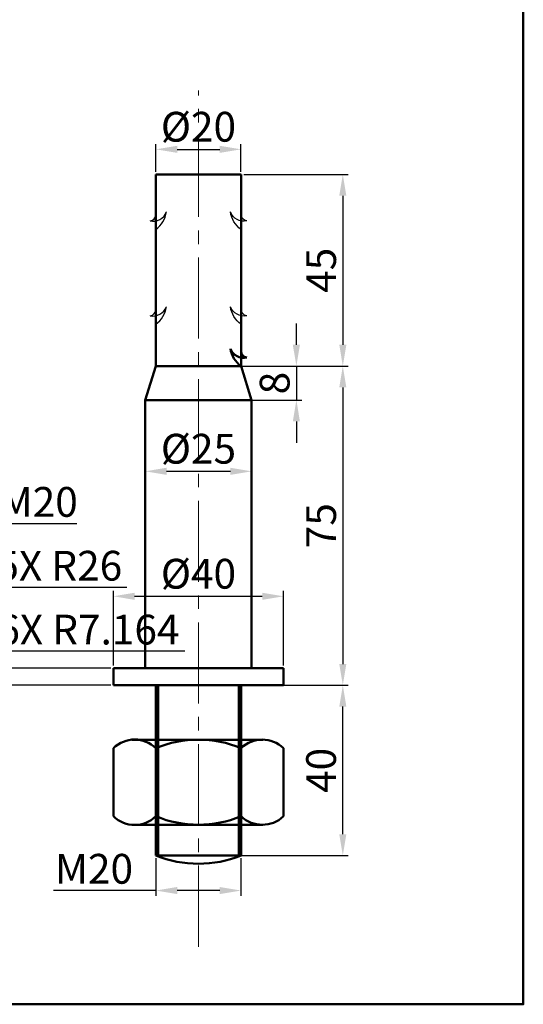
# Model space of a CAD drawing. Units: millimetres. Extents: x 120 to 482, y 299 to 766.
# Tile 2 of 3: x 355 to 473, y 299 to 531. Entities that reach past the tile are written whole.
import ezdxf

# ---------------------------------------------------------------- set-up
doc = ezdxf.new("R2010")
doc.units = ezdxf.units.MM
doc.linetypes.add('CENTER2', pattern=[28.575, 19.05, -3.175, 3.175, -3.175])
for name, color, linetype, lineweight in [('M-CNTR', 4, 'CENTER2', 18), ('M-DIMS', 2, 'Continuous', 25), ('M-OUTL', 7, 'Continuous', 50), ('M-SYMB', 7, 'Continuous', 25)]:
    doc.layers.add(name, color=color, linetype=linetype, lineweight=lineweight)
doc.styles.get("Standard").update_dxf_attribs({"font": 'arial.ttf'})
doc.dimstyles.new('ISO-25', dxfattribs={"dimtxt": 7, "dimasz": 5, "dimexe": 1.25, "dimexo": 0.625, "dimtad": 1, "dimtoh": 1, "dimdec": 0, "dimtxsty": 'Standard', "dimcen": 2.5, "dimadec": 0, "dimazin": 0, "dimtfac": 1, "dimtdec": 0, "dimtmove": 0, "dimatfit": 3, "dimfxl": 1, "dimarcsym": 0})

# ---------------------------------------------------------------- blocks, each defined once
blk = doc.blocks.new('*D3')
at = {"layer": 'Defpoints', "color": 0, "transparency": 16777216}
for p in [(342.61, 407.23), (342.61, 387.23), (349.55, 387.23)]:
    blk.add_point(p, dxfattribs=at)
at = {"layer": 'M-DIMS', "color": 0, "lineweight": -2, "transparency": 16777216}
for p, q in [((349.55, 407.23), (349.55, 412.23)), ((349.55, 412.23), (368, 412.23)), ((343.23, 407.23), (350.8, 407.23)), ((349.55, 392.23), (349.55, 402.23)), ((343.23, 387.23), (350.8, 387.23))]:
    blk.add_line(p, q, dxfattribs=at)
at = {"layer": 'M-DIMS', "color": 0, "transparency": 16777216}
for points in [[(348.72, 402.23), (350.38, 402.23), (349.55, 407.23)], [(348.72, 392.23), (350.38, 392.23), (349.55, 387.23)]]:
    blk.add_solid(points, dxfattribs=at)
at = {"layer": 'M-DIMS', "color": 0, "transparency": 16777216, "insert": (359.09, 416.43), "char_height": 7, "attachment_point": 5}
blk.add_mtext('M20', dxfattribs=at)
blk = doc.blocks.new('*U13')
at = {"layer": 'M-CNTR', "color": 0, "transparency": 16777216}
blk.add_line((0, -96.92), (0, 104.23), dxfattribs=at)
blk = doc.blocks.new('*D14')
at = {"layer": 'Defpoints', "color": 0, "transparency": 16777216}
for p in [(386.62, 334.25), (406.62, 334.25), (406.62, 326.03)]:
    blk.add_point(p, dxfattribs=at)
at = {"layer": 'M-DIMS', "color": 0, "lineweight": -2, "transparency": 16777216}
for p, q in [((386.62, 333.62), (386.62, 324.78)), ((406.62, 333.62), (406.62, 324.78)), ((386.62, 326.03), (362.55, 326.03)), ((401.62, 326.03), (391.62, 326.03))]:
    blk.add_line(p, q, dxfattribs=at)
at = {"layer": 'M-DIMS', "color": 0, "transparency": 16777216}
for points in [[(391.62, 326.86), (391.62, 325.19), (386.62, 326.03)], [(401.62, 326.86), (401.62, 325.19), (406.62, 326.03)]]:
    blk.add_solid(points, dxfattribs=at)
at = {"layer": 'M-DIMS', "color": 0, "transparency": 16777216, "insert": (372.08, 330.23), "char_height": 7, "attachment_point": 5}
blk.add_mtext('M20', dxfattribs=at)
blk = doc.blocks.new('*D15')
at = {"layer": 'Defpoints', "color": 0, "transparency": 16777216}
for p in [(396.62, 374.25), (430.55, 374.25), (396.62, 334.25)]:
    blk.add_point(p, dxfattribs=at)
at = {"layer": 'M-DIMS', "color": 0, "lineweight": -2, "transparency": 16777216}
for p, q in [((397.25, 374.25), (431.8, 374.25)), ((430.55, 339.25), (430.55, 369.25)), ((397.25, 334.25), (431.8, 334.25))]:
    blk.add_line(p, q, dxfattribs=at)
at = {"layer": 'M-DIMS', "color": 0, "transparency": 16777216}
for points in [[(429.72, 369.25), (431.38, 369.25), (430.55, 374.25)], [(429.72, 339.25), (431.38, 339.25), (430.55, 334.25)]]:
    blk.add_solid(points, dxfattribs=at)
at = {"layer": 'M-DIMS', "color": 0, "transparency": 16777216, "insert": (426.35, 354.25), "char_height": 7, "attachment_point": 5, "rotation": 90}
blk.add_mtext('40', dxfattribs=at)
blk = doc.blocks.new('*D16')
at = {"layer": 'Defpoints', "color": 0, "transparency": 16777216}
for p in [(416.62, 395.16), (376.62, 378.25), (416.62, 378.25)]:
    blk.add_point(p, dxfattribs=at)
at = {"layer": 'M-DIMS', "color": 0, "lineweight": -2, "transparency": 16777216}
for p, q in [((376.62, 378.87), (376.62, 396.41)), ((416.62, 378.87), (416.62, 396.41)), ((381.62, 395.16), (411.62, 395.16))]:
    blk.add_line(p, q, dxfattribs=at)
at = {"layer": 'M-DIMS', "color": 0, "transparency": 16777216}
for points in [[(381.62, 395.99), (381.62, 394.32), (376.62, 395.16)], [(411.62, 395.99), (411.62, 394.32), (416.62, 395.16)]]:
    blk.add_solid(points, dxfattribs=at)
at = {"layer": 'M-DIMS', "color": 0, "transparency": 16777216, "insert": (396.62, 399.55), "char_height": 7, "attachment_point": 5}
blk.add_mtext('%%C40', dxfattribs=at)
blk = doc.blocks.new('*D17')
at = {"layer": 'Defpoints', "color": 0, "transparency": 16777216}
for p in [(384.12, 423.55), (409.12, 424.52), (409.12, 423.55)]:
    blk.add_point(p, dxfattribs=at)
at = {"layer": 'M-DIMS', "color": 0, "lineweight": -2, "transparency": 16777216}
for p, q in [((384.12, 424.18), (384.12, 425.77)), ((409.12, 424.18), (409.12, 425.77)), ((389.12, 424.52), (404.12, 424.52))]:
    blk.add_line(p, q, dxfattribs=at)
at = {"layer": 'M-DIMS', "color": 0, "transparency": 16777216}
for points in [[(389.12, 425.36), (389.12, 423.69), (384.12, 424.52)], [(404.12, 425.36), (404.12, 423.69), (409.12, 424.52)]]:
    blk.add_solid(points, dxfattribs=at)
at = {"layer": 'M-DIMS', "color": 0, "transparency": 16777216, "insert": (396.62, 428.92), "char_height": 7, "attachment_point": 5}
blk.add_mtext('%%C25', dxfattribs=at)
blk = doc.blocks.new('*D18')
at = {"layer": 'Defpoints', "color": 0, "transparency": 16777216}
for p in [(396.62, 449.25), (396.62, 441.25), (419.64, 441.25)]:
    blk.add_point(p, dxfattribs=at)
at = {"layer": 'M-DIMS', "color": 0, "lineweight": -2, "transparency": 16777216}
for p, q in [((419.64, 454.25), (419.64, 459.25)), ((397.25, 449.25), (420.89, 449.25)), ((419.64, 449.25), (419.64, 441.25)), ((397.25, 441.25), (420.89, 441.25)), ((419.64, 436.25), (419.64, 431.25))]:
    blk.add_line(p, q, dxfattribs=at)
at = {"layer": 'M-DIMS', "color": 0, "transparency": 16777216}
for points in [[(418.8, 454.25), (420.47, 454.25), (419.64, 449.25)], [(418.8, 436.25), (420.47, 436.25), (419.64, 441.25)]]:
    blk.add_solid(points, dxfattribs=at)
at = {"layer": 'M-DIMS', "color": 0, "transparency": 16777216, "insert": (415.44, 445.25), "char_height": 7, "attachment_point": 5, "rotation": 90}
blk.add_mtext('8', dxfattribs=at)
blk = doc.blocks.new('*D19')
at = {"layer": 'Defpoints', "color": 0, "transparency": 16777216}
for p in [(406.62, 494.25), (396.62, 449.25), (430.55, 449.25)]:
    blk.add_point(p, dxfattribs=at)
at = {"layer": 'M-DIMS', "color": 0, "lineweight": -2, "transparency": 16777216}
for p, q in [((407.25, 494.25), (431.8, 494.25)), ((430.55, 489.25), (430.55, 454.25)), ((397.25, 449.25), (431.8, 449.25))]:
    blk.add_line(p, q, dxfattribs=at)
at = {"layer": 'M-DIMS', "color": 0, "transparency": 16777216}
for points in [[(429.72, 489.25), (431.38, 489.25), (430.55, 494.25)], [(429.72, 454.25), (431.38, 454.25), (430.55, 449.25)]]:
    blk.add_solid(points, dxfattribs=at)
at = {"layer": 'M-DIMS', "color": 0, "transparency": 16777216, "insert": (426.36, 471.75), "char_height": 7, "attachment_point": 5, "rotation": 90}
blk.add_mtext('45', dxfattribs=at)
blk = doc.blocks.new('*D20')
at = {"layer": 'Defpoints', "color": 0, "transparency": 16777216}
for p in [(424.07, 449.25), (424.07, 374.25), (430.55, 374.25)]:
    blk.add_point(p, dxfattribs=at)
at = {"layer": 'M-DIMS', "color": 0, "lineweight": -2, "transparency": 16777216}
for p, q in [((424.69, 449.25), (431.8, 449.25)), ((430.55, 444.25), (430.55, 379.25)), ((424.69, 374.25), (431.8, 374.25))]:
    blk.add_line(p, q, dxfattribs=at)
at = {"layer": 'M-DIMS', "color": 0, "transparency": 16777216}
for points in [[(429.72, 444.25), (431.38, 444.25), (430.55, 449.25)], [(429.72, 379.25), (431.38, 379.25), (430.55, 374.25)]]:
    blk.add_solid(points, dxfattribs=at)
at = {"layer": 'M-DIMS', "color": 0, "transparency": 16777216, "insert": (426.36, 411.75), "char_height": 7, "attachment_point": 5, "rotation": 90}
blk.add_mtext('75', dxfattribs=at)
blk = doc.blocks.new('*D21')
at = {"layer": 'Defpoints', "color": 0, "transparency": 16777216}
for p in [(406.62, 500.17), (386.62, 494.25), (406.62, 494.25)]:
    blk.add_point(p, dxfattribs=at)
at = {"layer": 'M-DIMS', "color": 0, "lineweight": -2, "transparency": 16777216}
for p, q in [((386.62, 494.87), (386.62, 501.42)), ((391.62, 500.17), (401.62, 500.17)), ((406.62, 494.87), (406.62, 501.42))]:
    blk.add_line(p, q, dxfattribs=at)
at = {"layer": 'M-DIMS', "color": 0, "transparency": 16777216}
for points in [[(391.62, 501), (391.62, 499.34), (386.62, 500.17)], [(401.62, 501), (401.62, 499.34), (406.62, 500.17)]]:
    blk.add_solid(points, dxfattribs=at)
at = {"layer": 'M-DIMS', "color": 0, "transparency": 16777216, "insert": (396.62, 504.57), "char_height": 7, "attachment_point": 5}
blk.add_mtext('%%C20', dxfattribs=at)
blk = doc.blocks.new('BREAK-MARK')
for centre, radius, start, end in [((0.72, 5.29), 3.36, 257.6696, 339.1974), ((-0.14, 3.52), 1.52, 275.355, 359.209), ((-2.21, 4.97), 6.13, 305.8281, 351.7873)]:
    blk.add_arc(centre, radius, start, end)
blk = doc.blocks.new('*D42')
at = {"layer": 'Defpoints', "color": 0, "transparency": 16777216}
for p in [(376.62, 378.25), (149.13, 374.25), (376.62, 374.25)]:
    blk.add_point(p, dxfattribs=at)
at = {"layer": 'M-DIMS', "color": 0, "lineweight": -2, "transparency": 16777216}
for p, q in [((149.13, 383.25), (149.13, 388.25)), ((376, 378.25), (147.88, 378.25)), ((149.13, 378.25), (149.13, 374.25)), ((376, 374.25), (147.88, 374.25)), ((149.13, 369.25), (149.13, 364.25)), ((149.13, 364.25), (143.66, 364.25))]:
    blk.add_line(p, q, dxfattribs=at)
at = {"layer": 'M-DIMS', "color": 0, "transparency": 16777216}
for points in [[(148.29, 383.25), (149.96, 383.25), (149.13, 378.25)], [(148.29, 369.25), (149.96, 369.25), (149.13, 374.25)]]:
    blk.add_solid(points, dxfattribs=at)
at = {"layer": 'M-DIMS', "color": 0, "transparency": 16777216, "insert": (146.08, 368.37), "char_height": 7, "attachment_point": 5}
blk.add_mtext('4', dxfattribs=at)
blk = doc.blocks.new('*D44')
at = {"layer": 'Defpoints', "color": 0, "transparency": 16777216}
for p in [(304.27, 397.23), (330.27, 397.23)]:
    blk.add_point(p, dxfattribs=at)
at = {"layer": 'M-DIMS', "color": 0, "lineweight": -2, "transparency": 16777216}
for p, q in [((304.27, 397.23), (330.27, 397.23)), ((347.42, 397.23), (335.27, 397.23)), ((379.8, 397.23), (347.42, 397.23))]:
    blk.add_line(p, q, dxfattribs=at)
at = {"layer": 'M-DIMS', "color": 0, "transparency": 16777216}
blk.add_solid([(335.27, 398.06), (335.27, 396.4), (330.27, 397.23)], dxfattribs=at)
at = {"layer": 'M-DIMS', "color": 0, "transparency": 16777216, "insert": (363.92, 401.43), "char_height": 7, "attachment_point": 5}
blk.add_mtext('5X R26', dxfattribs=at)
blk = doc.blocks.new('*D46')
at = {"layer": 'Defpoints', "color": 0, "transparency": 16777216}
for p in [(323.14, 382.23), (330.3, 382.23)]:
    blk.add_point(p, dxfattribs=at)
at = {"layer": 'M-DIMS', "color": 0, "lineweight": -2, "transparency": 16777216}
for p, q in [((323.14, 382.23), (330.3, 382.23)), ((347.45, 382.23), (335.3, 382.23)), ((393.45, 382.23), (347.45, 382.23))]:
    blk.add_line(p, q, dxfattribs=at)
at = {"layer": 'M-DIMS', "color": 0, "transparency": 16777216}
blk.add_solid([(335.3, 383.06), (335.3, 381.4), (330.3, 382.23)], dxfattribs=at)
at = {"layer": 'M-DIMS', "color": 0, "transparency": 16777216, "insert": (370.76, 386.43), "char_height": 7, "attachment_point": 5}
blk.add_mtext('6X R7.164', dxfattribs=at)

msp = doc.modelspace()

# ---------------------------------------------------------------- linework, layer by layer
at = {"layer": 'M-OUTL'}
for p, q in [((406.6246, 494.2458), (386.6246, 494.2458)), ((386.6246, 494.2458), (386.6246, 449.2458)), ((406.6246, 449.2458), (406.6246, 494.2458)), ((386.6246, 449.2458), (384.1246, 441.2458)), ((386.6246, 449.2458), (406.6246, 449.2458)), ((406.6246, 449.2458), (409.1246, 441.2458)), ((384.1246, 441.2458), (409.1246, 441.2458)), ((384.1246, 378.2458), (384.1246, 441.2458)), ((409.1246, 378.2458), (409.1246, 441.2458)), ((386.6246, 374.2458), (406.6246, 374.2458)), ((386.6246, 374.2458), (386.6246, 334.2458)), ((387.1246, 374.2458), (387.1246, 334.2458)), ((406.1246, 374.2458), (406.1246, 334.2458)), ((406.6246, 334.2458), (406.6246, 374.2458)), ((411.7447, 361.4737), (380.9333, 361.4737)), ((376.6246, 359.4737), (376.6246, 343.4737)), ((386.6246, 359.4737), (386.6246, 343.4737)), ((406.6246, 341.4737), (406.6246, 359.4737)), ((416.6246, 343.4737), (416.6246, 359.4737)), ((380.9333, 341.4737), (411.7447, 341.4737)), ((386.6246, 334.2458), (406.6246, 334.2458))]:
    msp.add_line(p, q, dxfattribs=at)
msp.add_lwpolyline([(129.5751, 766.022), (472.9721, 766.022), (472.9721, 299.2966), (129.5751, 299.2966)], close=True, dxfattribs=at)
for centre, radius, start, end in [((407.2881, 454.5326), 3.3607, 200.802598, 282.33044), ((410.2119, 454.2145), 6.1283, 188.212732, 234.171857), ((408.1479, 452.7662), 1.5235, 180.791034, 264.644968), ((381.6246, 354.3432), 7.1639, 45.738071, 134.261929), ((396.6246, 335.4737), 26, 67.380135, 112.619865), ((411.6246, 354.2273), 7.2474, 46.377545, 133.622455), ((381.6246, 348.6042), 7.1639, 225.738071, 314.261929), ((396.6246, 367.4737), 26, 247.380135, 292.619865), ((411.6246, 348.7201), 7.2474, 226.377545, 313.622455), ((396.6246, 359.2234), 26.905, 248.180848, 291.819152)]:
    msp.add_arc(centre, radius, start, end, dxfattribs=at)
msp.add_open_spline([(416.6246, 378.2458), (416.458, 378.2458), (416.2913, 378.2458), (416.1246, 378.2458), (403.1246, 378.2458), (390.1246, 378.2458), (377.1246, 378.2458), (376.958, 378.2458), (376.7913, 378.2458), (376.6246, 378.2458)], degree=3, knots=[-0.01282051, -0.01282051, -0.01282051, -0.01282051, 0, 0, 0, 1, 1, 1, 2, 2, 2, 2], dxfattribs=at)
for points in [[(376.6246, 378.2458), (376.6246, 376.9125), (376.6246, 375.5791), (376.6246, 374.2458)], [(416.6246, 374.2458), (416.6246, 375.5791), (416.6246, 376.9125), (416.6246, 378.2458)], [(376.6246, 374.2458), (389.958, 374.2458), (403.2913, 374.2458), (416.6246, 374.2458)]]:
    msp.add_open_spline(points, degree=3, dxfattribs=at)

# ---------------------------------------------------------------- block references
at = {"layer": 'M-CNTR'}
msp.add_blockref('*U13', (396.6246, 409.7458), dxfattribs=at)
at = {"layer": 'M-SYMB'}
for p in [(385.243, 481.3577), (385.243, 459.081)]:
    msp.add_blockref('BREAK-MARK', p, dxfattribs=at)
at = {"layer": 'M-SYMB', "extrusion": (0, 0, -1), "zscale": -1}
for p in [(-408.0063, 481.3577), (-408.0063, 459.081)]:
    msp.add_blockref('BREAK-MARK', p, dxfattribs=at)

# ---------------------------------------------------------------- dimensions: what is measured, and where the dimension line sits
at = {"layer": 'M-DIMS'}
for base, p1, p2, picture, middle in [((406.6246, 500.171), (386.6246, 494.2458), (406.6246, 494.2458), '*D21', (396.6246, 504.5658)), ((409.1246, 424.5231), (384.1246, 423.5507), (409.1246, 423.5507), '*D17', (396.6246, 428.9179)), ((416.6246, 395.1577), (376.6246, 378.2458), (416.6246, 378.2458), '*D16', (396.6246, 399.5525))]:
    dim = msp.add_linear_dim(base=base, p1=p1, p2=p2, text='%%C<>', dimstyle='ISO-25', override={"dimclrd": 0, "dimclre": 0, "dimclrt": 0}, dxfattribs=at)
    dim.commit()
    dim.dimension.update_dxf_attribs({"geometry": picture, "text_midpoint": middle})
for base, p1, p2, override, picture, middle in [((430.5494, 449.2458), (406.6246, 494.2458), (396.6246, 449.2458), {"dimclrd": 0, "dimclre": 0, "dimclrt": 0}, '*D19', (426.3647, 471.7458)), ((419.6378, 441.2458), (396.6246, 449.2458), (396.6246, 441.2458), {"dimclrd": 0, "dimclre": 0, "dimclrt": 0}, '*D18', (415.4388, 445.2458)), ((430.5494, 374.2458), (424.0677, 449.2458), (424.0677, 374.2458), {"dimclrd": 0, "dimclre": 0, "dimclrt": 0}, '*D20', (426.3647, 411.7458)), ((149.1271, 374.2458), (376.6246, 378.2458), (376.6246, 374.2458), {"dimdec": 0, "dimlfac": 1, "dimrnd": 0, "dimzin": 0, "dimdsep": 46, "dimlunit": 2}, '*D42', (146.0812, 368.3708)), ((430.5494, 374.2458), (396.6246, 334.2458), (396.6246, 374.2458), {"dimclrd": 0, "dimclre": 0, "dimclrt": 0}, '*D15', (426.3504, 354.2458))]:
    dim = msp.add_linear_dim(base=base, p1=p1, p2=p2, angle=90, dimstyle='ISO-25', override=override, dxfattribs=at)
    dim.commit()
    dim.dimension.update_dxf_attribs({"geometry": picture, "text_midpoint": middle})
dim = msp.add_linear_dim(base=(349.5499, 387.2311), p1=(342.61, 407.2311), p2=(342.61, 387.2311), angle=90, text='M<>', dimstyle='ISO-25', override={"dimclrd": 0, "dimclre": 0, "dimclrt": 0}, dxfattribs=at)
dim.commit()
dim.dimension.update_dxf_attribs({"geometry": '*D3', "text_midpoint": (359.0896, 412.2311), "dimtype": 160})
for center, mpoint, text, override, picture, middle in [((304.2686, 397.2311), (330.2686, 397.231), '5X <>', {"dimdec": 0, "dimlfac": 1, "dimrnd": 0, "dimzin": 0, "dimdsep": 46, "dimlunit": 2}, '*D44', (363.9229, 401.43)), ((323.1381, 382.2311), (330.302, 382.231), '6X <>', {"dimdec": 3, "dimlfac": 1, "dimrnd": 0, "dimzin": 0, "dimdsep": 46, "dimlunit": 2}, '*D46', (370.7606, 386.4298))]:
    dim = msp.add_radius_dim(center=center, mpoint=mpoint, text=text, dimstyle='ISO-25', override=override, dxfattribs=at)
    dim.commit()
    dim.dimension.update_dxf_attribs({"geometry": picture, "text_midpoint": middle})
dim = msp.add_linear_dim(base=(406.6246, 326.0275), p1=(386.6246, 334.2458), p2=(406.6246, 334.2458), text='M<>', dimstyle='ISO-25', override={"dimclrd": 0, "dimclre": 0, "dimclrt": 0}, dxfattribs=at)
dim.commit()
dim.dimension.update_dxf_attribs({"geometry": '*D14', "text_midpoint": (372.0849, 326.0275), "dimtype": 160})

doc.saveas('drawing.dxf')
